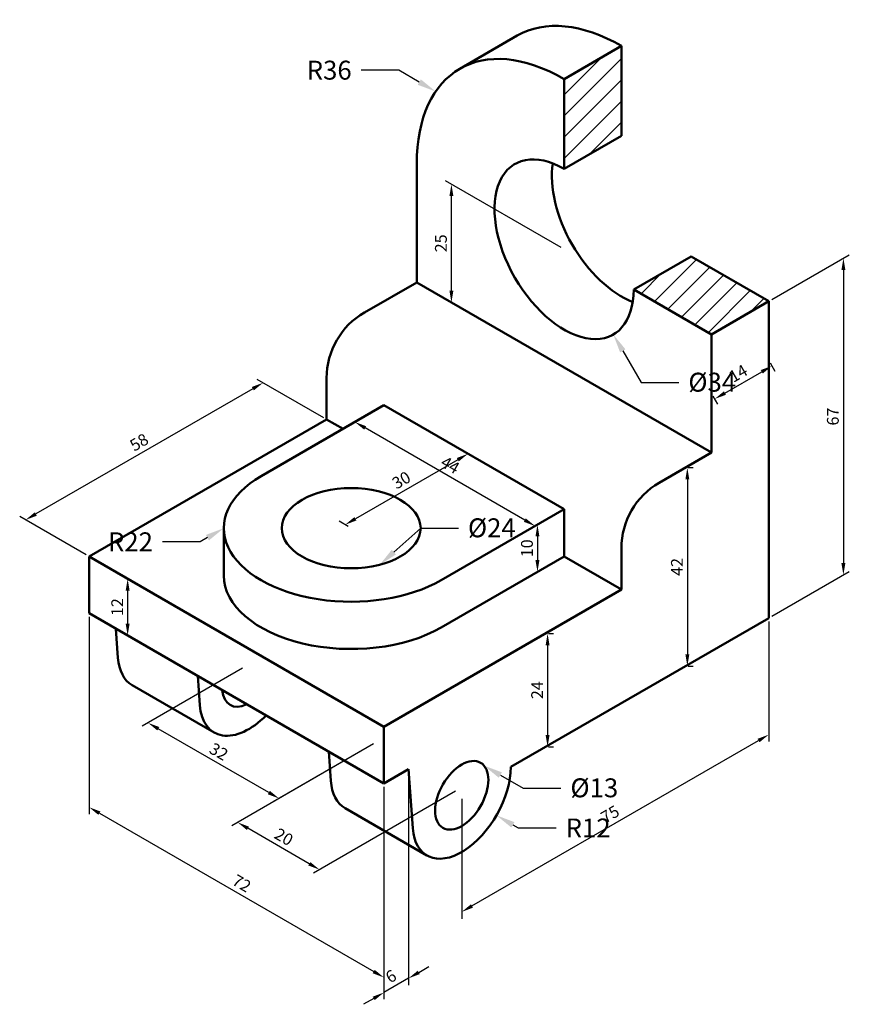
# Model space of a CAD drawing. Units: millimetres. Extents: x 4591 to 4766, y 1465 to 1673.
import ezdxf
from ezdxf import colors
from ezdxf.entities.mleader import LeaderData, LeaderLine
from ezdxf.math import Vec2, Vec3

# ---------------------------------------------------------------- set-up
doc = ezdxf.new("R2010")
doc.units = ezdxf.units.MM
for name, color, linetype, lineweight in [('M-DIMS', 2, 'Continuous', 25), ('M-HATC', 8, 'Continuous', 18), ('M-OUTL', 7, 'Continuous', 50), ('M-TEXT', 3, 'Continuous', 25)]:
    doc.layers.add(name, color=color, linetype=linetype, lineweight=lineweight)
doc.styles.get("Standard").update_dxf_attribs({"font": 'arial.ttf'})
doc.dimstyles.new('ISO-25', dxfattribs={"dimtxt": 2.5, "dimasz": 2.5, "dimexe": 1.25, "dimexo": 0.625, "dimtad": 1, "dimtxsty": 'Standard', "dimcen": 2.5, "dimadec": 0, "dimazin": 0, "dimtfac": 1, "dimtmove": 0, "dimatfit": 3, "dimfxl": 1, "dimarcsym": 0})

# ---------------------------------------------------------------- blocks, each defined once
blk = doc.blocks.new('*D1')
at = {"layer": 'Defpoints', "color": 0, "transparency": 16777216}
for p in [(4749.17, 1546.38), (4749.17, 1521.72), (4684.22, 1508.88)]:
    blk.add_point(p, dxfattribs=at)
at = {"layer": 'M-DIMS', "color": 0, "lineweight": -2, "transparency": 16777216}
for p, q in [((4749.17, 1545.66), (4749.17, 1520.27)), ((4686.39, 1485.47), (4747.01, 1520.47)), ((4684.22, 1508.16), (4684.22, 1482.77))]:
    blk.add_line(p, q, dxfattribs=at)
at = {"layer": 'M-DIMS', "color": 0, "transparency": 16777216}
for points in [[(4746.8, 1520.83), (4747.22, 1520.11), (4749.17, 1521.72)], [(4686.18, 1485.83), (4686.59, 1485.11), (4684.22, 1484.22)]]:
    blk.add_solid(points, dxfattribs=at)
at = {"layer": 'M-DIMS', "color": 0, "transparency": 16777216, "insert": (4715.75, 1504.61), "char_height": 2.5, "attachment_point": 5, "rotation": 30}
blk.add_mtext('75', dxfattribs=at)
blk = doc.blocks.new('*D2')
at = {"layer": 'Defpoints', "color": 0, "transparency": 16777216}
for p in [(4672.96, 1514.38), (4667.77, 1511.38), (4667.77, 1467.17)]:
    blk.add_point(p, dxfattribs=at)
at = {"layer": 'M-DIMS', "color": 0, "lineweight": -2, "transparency": 16777216}
for p, q in [((4672.96, 1513.66), (4672.96, 1468.73)), ((4667.77, 1510.66), (4667.77, 1465.73)), ((4675.13, 1471.42), (4677.29, 1472.67)), ((4672.96, 1470.17), (4667.77, 1467.17)), ((4665.6, 1465.92), (4663.44, 1464.67))]:
    blk.add_line(p, q, dxfattribs=at)
at = {"layer": 'M-DIMS', "color": 0, "transparency": 16777216}
for points in [[(4674.92, 1471.78), (4675.34, 1471.06), (4672.96, 1470.17)], [(4665.39, 1466.28), (4665.81, 1465.56), (4667.77, 1467.17)]]:
    blk.add_solid(points, dxfattribs=at)
at = {"layer": 'M-DIMS', "color": 0, "transparency": 16777216, "insert": (4669.41, 1470.32), "char_height": 2.5, "attachment_point": 5, "rotation": 30}
blk.add_mtext('6', dxfattribs=at)
blk = doc.blocks.new('*D3')
at = {"layer": 'Defpoints', "color": 0, "transparency": 16777216}
for p in [(4655.64, 1588.38), (4591.97, 1567.14), (4605.41, 1559.38)]:
    blk.add_point(p, dxfattribs=at)
at = {"layer": 'M-DIMS', "color": 0, "lineweight": -2, "transparency": 16777216}
for p, q in [((4655.02, 1588.74), (4640.95, 1596.86)), ((4640.04, 1594.89), (4594.14, 1568.39)), ((4604.79, 1559.74), (4590.72, 1567.86))]:
    blk.add_line(p, q, dxfattribs=at)
at = {"layer": 'M-DIMS', "color": 0, "transparency": 16777216}
for points in [[(4639.83, 1595.25), (4640.25, 1594.53), (4642.2, 1596.14)], [(4593.93, 1568.75), (4594.35, 1568.03), (4591.97, 1567.14)]]:
    blk.add_solid(points, dxfattribs=at)
at = {"layer": 'M-DIMS', "color": 0, "transparency": 16777216, "insert": (4616.14, 1583.29), "char_height": 2.5, "attachment_point": 5, "rotation": 30}
blk.add_mtext('58', dxfattribs=at)
blk = doc.blocks.new('*D4')
at = {"layer": 'Defpoints', "color": 0, "transparency": 16777216}
for p in [(4701.94, 1543.12), (4701.94, 1519.12), (4702.38, 1519.12)]:
    blk.add_point(p, dxfattribs=at)
at = {"layer": 'M-DIMS', "color": 0, "lineweight": -2, "transparency": 16777216}
for p, q in [((4702.57, 1543.12), (4703.63, 1543.12)), ((4702.38, 1540.62), (4702.38, 1521.62)), ((4702.57, 1519.12), (4703.63, 1519.12))]:
    blk.add_line(p, q, dxfattribs=at)
at = {"layer": 'M-DIMS', "color": 0, "transparency": 16777216}
for points in [[(4701.96, 1540.62), (4702.79, 1540.62), (4702.38, 1543.12)], [(4701.96, 1521.62), (4702.79, 1521.62), (4702.38, 1519.12)]]:
    blk.add_solid(points, dxfattribs=at)
at = {"layer": 'M-DIMS', "color": 0, "transparency": 16777216, "insert": (4700.5, 1531.12), "char_height": 2.5, "attachment_point": 5, "rotation": 90}
blk.add_mtext('24', dxfattribs=at)
blk = doc.blocks.new('*D5')
at = {"layer": 'Defpoints', "color": 0, "transparency": 16777216}
for p in [(4731.52, 1578.19), (4731.52, 1536.19), (4731.94, 1536.19)]:
    blk.add_point(p, dxfattribs=at)
at = {"layer": 'M-DIMS', "color": 0, "lineweight": -2, "transparency": 16777216}
for p, q in [((4732.15, 1578.19), (4733.19, 1578.19)), ((4731.94, 1575.69), (4731.94, 1538.69)), ((4732.15, 1536.19), (4733.19, 1536.19))]:
    blk.add_line(p, q, dxfattribs=at)
at = {"layer": 'M-DIMS', "color": 0, "transparency": 16777216}
for points in [[(4731.53, 1575.69), (4732.36, 1575.69), (4731.94, 1578.19)], [(4731.53, 1538.69), (4732.36, 1538.69), (4731.94, 1536.19)]]:
    blk.add_solid(points, dxfattribs=at)
at = {"layer": 'M-DIMS', "color": 0, "transparency": 16777216, "insert": (4730.06, 1557.19), "char_height": 2.5, "attachment_point": 5, "rotation": 90}
blk.add_mtext('42', dxfattribs=at)
blk = doc.blocks.new('*D6')
at = {"layer": 'Defpoints', "color": 0, "transparency": 16777216}
for p in [(4749.17, 1613.38), (4764.95, 1555.49), (4749.17, 1546.38)]:
    blk.add_point(p, dxfattribs=at)
at = {"layer": 'M-DIMS', "color": 0, "lineweight": -2, "transparency": 16777216}
for p, q in [((4749.8, 1613.74), (4766.2, 1623.21)), ((4764.95, 1619.99), (4764.95, 1557.99)), ((4749.8, 1546.74), (4766.2, 1556.21))]:
    blk.add_line(p, q, dxfattribs=at)
at = {"layer": 'M-DIMS', "color": 0, "transparency": 16777216}
for points in [[(4764.53, 1619.99), (4765.37, 1619.99), (4764.95, 1622.49)], [(4764.53, 1557.99), (4765.37, 1557.99), (4764.95, 1555.49)]]:
    blk.add_solid(points, dxfattribs=at)
at = {"layer": 'M-DIMS', "color": 0, "transparency": 16777216, "insert": (4763.05, 1588.99), "char_height": 2.5, "attachment_point": 5, "rotation": 90}
blk.add_mtext('67', dxfattribs=at)
blk = doc.blocks.new('*D7')
at = {"layer": 'Defpoints', "color": 0, "transparency": 16777216}
for p in [(4749.17, 1600.88), (4749.85, 1599.72), (4737.05, 1593.88)]:
    blk.add_point(p, dxfattribs=at)
at = {"layer": 'M-DIMS', "color": 0, "lineweight": -2, "transparency": 16777216}
for p, q in [((4749.49, 1600.34), (4750.47, 1598.63)), ((4739.89, 1593.97), (4747.68, 1598.47)), ((4737.36, 1593.34), (4738.35, 1591.63))]:
    blk.add_line(p, q, dxfattribs=at)
at = {"layer": 'M-DIMS', "color": 0, "transparency": 16777216}
for points in [[(4747.47, 1598.83), (4747.89, 1598.1), (4749.85, 1599.72)], [(4739.68, 1594.33), (4740.1, 1593.6), (4737.72, 1592.72)]]:
    blk.add_solid(points, dxfattribs=at)
at = {"layer": 'M-DIMS', "color": 0, "transparency": 16777216, "insert": (4742.85, 1597.84), "char_height": 2.5, "attachment_point": 5, "rotation": 30}
blk.add_mtext('14', dxfattribs=at)
blk = doc.blocks.new('*D8')
at = {"layer": 'Defpoints', "color": 0, "transparency": 16777216}
for p in [(4682.04, 1638.14), (4705.87, 1624.38), (4705.87, 1599.38)]:
    blk.add_point(p, dxfattribs=at)
at = {"layer": 'M-DIMS', "color": 0, "lineweight": -2, "transparency": 16777216}
for p, q in [((4705.25, 1624.74), (4680.79, 1638.86)), ((4682.04, 1615.64), (4682.04, 1635.64)), ((4705.25, 1599.74), (4680.79, 1613.86))]:
    blk.add_line(p, q, dxfattribs=at)
at = {"layer": 'M-DIMS', "color": 0, "transparency": 16777216}
for points in [[(4681.62, 1635.64), (4682.46, 1635.64), (4682.04, 1638.14)], [(4681.62, 1615.64), (4682.46, 1615.64), (4682.04, 1613.14)]]:
    blk.add_solid(points, dxfattribs=at)
at = {"layer": 'M-DIMS', "color": 0, "transparency": 16777216, "insert": (4680.14, 1625.64), "char_height": 2.5, "attachment_point": 5, "rotation": 90}
blk.add_mtext('25', dxfattribs=at)
blk = doc.blocks.new('*D9')
at = {"layer": 'Defpoints', "color": 0, "transparency": 16777216}
for p in [(4667.77, 1591.38), (4661.63, 1587.84), (4705.87, 1569.38)]:
    blk.add_point(p, dxfattribs=at)
at = {"layer": 'M-DIMS', "color": 0, "lineweight": -2, "transparency": 16777216}
for p, q in [((4667.14, 1591.02), (4660.38, 1587.12)), ((4697.57, 1567.09), (4663.8, 1586.59)), ((4705.25, 1569.02), (4698.49, 1565.12))]:
    blk.add_line(p, q, dxfattribs=at)
at = {"layer": 'M-DIMS', "color": 0, "transparency": 16777216}
for points in [[(4664.01, 1586.95), (4663.59, 1586.23), (4661.63, 1587.84)], [(4697.78, 1567.45), (4697.37, 1566.73), (4699.74, 1565.84)]]:
    blk.add_solid(points, dxfattribs=at)
at = {"layer": 'M-DIMS', "color": 0, "transparency": 16777216, "insert": (4681.62, 1578.47), "char_height": 2.5, "attachment_point": 5, "rotation": 330}
blk.add_mtext('44', dxfattribs=at)
blk = doc.blocks.new('*D10')
at = {"layer": 'Defpoints', "color": 0, "transparency": 16777216}
for p in [(4705.87, 1569.38), (4705.87, 1559.38), (4700.24, 1556.13)]:
    blk.add_point(p, dxfattribs=at)
at = {"layer": 'M-DIMS', "color": 0, "lineweight": -2, "transparency": 16777216}
for p, q in [((4705.25, 1569.02), (4698.99, 1565.41)), ((4700.24, 1563.63), (4700.24, 1558.63)), ((4705.25, 1559.02), (4698.99, 1555.41))]:
    blk.add_line(p, q, dxfattribs=at)
at = {"layer": 'M-DIMS', "color": 0, "transparency": 16777216}
for points in [[(4699.82, 1563.63), (4700.65, 1563.63), (4700.24, 1566.13)], [(4699.82, 1558.63), (4700.65, 1558.63), (4700.24, 1556.13)]]:
    blk.add_solid(points, dxfattribs=at)
at = {"layer": 'M-DIMS', "color": 0, "transparency": 16777216, "insert": (4698.34, 1561.13), "char_height": 2.5, "attachment_point": 5, "rotation": 90}
blk.add_mtext('10', dxfattribs=at)
blk = doc.blocks.new('*D11')
at = {"layer": 'Defpoints', "color": 0, "transparency": 16777216}
for p in [(4686.82, 1580.38), (4659.57, 1566.12), (4660.84, 1565.38)]:
    blk.add_point(p, dxfattribs=at)
at = {"layer": 'M-DIMS', "color": 0, "lineweight": -2, "transparency": 16777216}
for p, q in [((4686.19, 1580.74), (4684.3, 1581.84)), ((4683.38, 1579.87), (4661.73, 1567.37)), ((4660.21, 1565.74), (4658.32, 1566.84))]:
    blk.add_line(p, q, dxfattribs=at)
at = {"layer": 'M-DIMS', "color": 0, "transparency": 16777216}
for points in [[(4683.17, 1580.23), (4683.59, 1579.51), (4685.55, 1581.12)], [(4661.52, 1567.73), (4661.94, 1567.01), (4659.57, 1566.12)]]:
    blk.add_solid(points, dxfattribs=at)
at = {"layer": 'M-DIMS', "color": 0, "transparency": 16777216, "insert": (4671.6, 1575.27), "char_height": 2.5, "attachment_point": 5, "rotation": 30}
blk.add_mtext('30', dxfattribs=at)
blk = doc.blocks.new('*D12')
at = {"layer": 'Defpoints', "color": 0, "transparency": 16777216}
for p in [(4605.41, 1547.38), (4667.77, 1511.38), (4667.77, 1470.35)]:
    blk.add_point(p, dxfattribs=at)
at = {"layer": 'M-DIMS', "color": 0, "lineweight": -2, "transparency": 16777216}
for p, q in [((4605.41, 1546.66), (4605.41, 1504.91)), ((4667.77, 1510.66), (4667.77, 1468.91)), ((4607.58, 1505.1), (4665.6, 1471.6))]:
    blk.add_line(p, q, dxfattribs=at)
at = {"layer": 'M-DIMS', "color": 0, "transparency": 16777216}
for points in [[(4607.79, 1505.46), (4607.37, 1504.74), (4605.41, 1506.35)], [(4665.81, 1471.96), (4665.39, 1471.24), (4667.77, 1470.35)]]:
    blk.add_solid(points, dxfattribs=at)
at = {"layer": 'M-DIMS', "color": 0, "transparency": 16777216, "insert": (4637.53, 1489.98), "char_height": 2.5, "attachment_point": 5, "rotation": 330}
blk.add_mtext('72', dxfattribs=at)
blk = doc.blocks.new('*D13')
at = {"layer": 'Defpoints', "color": 0, "transparency": 16777216}
for p in [(4666.19, 1520.11), (4683.52, 1510.11), (4636.83, 1503.15)]:
    blk.add_point(p, dxfattribs=at)
at = {"layer": 'M-DIMS', "color": 0, "lineweight": -2, "transparency": 16777216}
for p, q in [((4665.57, 1519.75), (4635.58, 1502.43)), ((4682.89, 1509.75), (4652.9, 1492.43)), ((4651.98, 1494.4), (4638.99, 1501.9))]:
    blk.add_line(p, q, dxfattribs=at)
at = {"layer": 'M-DIMS', "color": 0, "transparency": 16777216}
for points in [[(4639.2, 1502.26), (4638.78, 1501.54), (4636.83, 1503.15)], [(4652.19, 1494.76), (4651.77, 1494.04), (4654.15, 1493.15)]]:
    blk.add_solid(points, dxfattribs=at)
at = {"layer": 'M-DIMS', "color": 0, "transparency": 16777216, "insert": (4646.44, 1499.8), "char_height": 2.5, "attachment_point": 5, "rotation": 330}
blk.add_mtext('20', dxfattribs=at)
blk = doc.blocks.new('*D14')
at = {"layer": 'Defpoints', "color": 0, "transparency": 16777216}
for p in [(4638.48, 1536.11), (4617.87, 1524.21), (4666.19, 1520.11)]:
    blk.add_point(p, dxfattribs=at)
at = {"layer": 'M-DIMS', "color": 0, "lineweight": -2, "transparency": 16777216}
for p, q in [((4637.86, 1535.75), (4616.62, 1523.49)), ((4643.42, 1509.46), (4620.04, 1522.96)), ((4665.57, 1519.75), (4644.34, 1507.49))]:
    blk.add_line(p, q, dxfattribs=at)
at = {"layer": 'M-DIMS', "color": 0, "transparency": 16777216}
for points in [[(4620.25, 1523.32), (4619.83, 1522.6), (4617.87, 1524.21)], [(4643.63, 1509.82), (4643.21, 1509.1), (4645.59, 1508.21)]]:
    blk.add_solid(points, dxfattribs=at)
at = {"layer": 'M-DIMS', "color": 0, "transparency": 16777216, "insert": (4632.68, 1517.85), "char_height": 2.5, "attachment_point": 5, "rotation": 330}
blk.add_mtext('32', dxfattribs=at)
blk = doc.blocks.new('*D15')
at = {"layer": 'Defpoints', "color": 0, "transparency": 16777216}
for p in [(4621.72, 1549.97), (4613.56, 1542.68), (4621.72, 1537.97)]:
    blk.add_point(p, dxfattribs=at)
at = {"layer": 'M-DIMS', "color": 0, "lineweight": -2, "transparency": 16777216}
for p, q in [((4621.09, 1550.33), (4612.31, 1555.4)), ((4613.56, 1552.18), (4613.56, 1545.18)), ((4621.09, 1538.33), (4612.31, 1543.4))]:
    blk.add_line(p, q, dxfattribs=at)
at = {"layer": 'M-DIMS', "color": 0, "transparency": 16777216}
for points in [[(4613.14, 1552.18), (4613.97, 1552.18), (4613.56, 1554.68)], [(4613.14, 1545.18), (4613.97, 1545.18), (4613.56, 1542.68)]]:
    blk.add_solid(points, dxfattribs=at)
at = {"layer": 'M-DIMS', "color": 0, "transparency": 16777216, "insert": (4611.68, 1548.68), "char_height": 2.5, "attachment_point": 5, "rotation": 90}
blk.add_mtext('12', dxfattribs=at)

msp = doc.modelspace()

# ---------------------------------------------------------------- hatches: boundary and pattern name
at = {"layer": 'M-HATC'}
h = msp.add_hatch(dxfattribs=at)
h.set_pattern_fill('ANSI31', color=256)
h.paths.add_polyline_path([(4717.996, 1667.383), (4705.872, 1660.383), (4705.872, 1641.383), (4717.996, 1648.383)])
h.paths.add_polyline_path([(4749.173, 1613.383), (4732.719, 1622.883), (4720.595, 1615.883), (4737.049, 1606.383)])

# ---------------------------------------------------------------- linework, layer by layer
at = {"layer": 'M-OUTL'}
for p, q in [((4695.951, 1669.567), (4683.827, 1662.567)), ((4705.872, 1660.383), (4717.996, 1667.383)), ((4717.996, 1648.383), (4717.996, 1667.383)), ((4705.872, 1641.383), (4705.872, 1660.383)), ((4705.872, 1641.383), (4717.996, 1648.383)), ((4674.695, 1642.383), (4674.695, 1617.383)), ((4720.595, 1615.883), (4732.719, 1622.883)), ((4732.719, 1622.883), (4749.173, 1613.383)), ((4674.695, 1617.383), (4663.643, 1611.002)), ((4674.695, 1617.383), (4737.049, 1581.383)), ((4720.595, 1615.883), (4737.049, 1606.383)), ((4749.173, 1613.383), (4737.049, 1606.383)), ((4749.173, 1546.383), (4749.173, 1613.383)), ((4737.049, 1606.383), (4737.049, 1581.383)), ((4655.643, 1597.145), (4655.643, 1588.383)), ((4641.786, 1576.383), (4667.767, 1591.383)), ((4705.872, 1569.383), (4667.767, 1591.383)), ((4655.643, 1588.383), (4605.413, 1559.383)), ((4659.107, 1586.383), (4655.643, 1588.383)), ((4737.049, 1581.383), (4725.996, 1575.002)), ((4679.891, 1554.383), (4705.872, 1569.383)), ((4705.872, 1559.383), (4705.872, 1569.383)), ((4633.894, 1565.383), (4633.894, 1555.383)), ((4717.996, 1561.145), (4717.996, 1552.383)), ((4605.413, 1559.383), (4605.413, 1547.383)), ((4605.413, 1559.383), (4667.767, 1523.383)), ((4705.872, 1559.383), (4679.891, 1544.383)), ((4717.996, 1552.383), (4705.872, 1559.383)), ((4717.996, 1552.383), (4667.767, 1523.383)), ((4605.413, 1547.383), (4667.767, 1511.383)), ((4749.173, 1546.383), (4694.614, 1514.883)), ((4611.062, 1544.122), (4611.509, 1537.944)), ((4628.382, 1534.122), (4628.829, 1527.944)), ((4614.519, 1532.155), (4631.84, 1522.155)), ((4667.767, 1523.383), (4667.767, 1511.383)), ((4656.095, 1518.122), (4656.542, 1511.944)), ((4667.767, 1511.383), (4672.963, 1514.383)), ((4672.963, 1514.383), (4673.862, 1501.944)), ((4659.552, 1506.155), (4676.873, 1496.155))]:
    msp.add_line(p, q, dxfattribs=at)
for centre in [(4671.643, 1597.145), (4733.996, 1561.145)]:
    msp.add_arc(centre, 16, 120, 180, dxfattribs=at)
for centre, major_axis, start_param, end_param in [((4717.996, 1631.383), (22.045, -38.184), 8.6393798, 9.424778), ((4705.872, 1624.383), (22.045, -38.184), 8.6393798, 10.2101761), ((4705.872, 1624.383), (10.41, -18.031), 2.3561945, 7.0685835), ((4717.996, 1631.383), (10.41, -18.031), 3.7631762, 5.6616018), ((4660.839, 1565.383), (-26.944, 0), 5.4977871, 8.6393798), ((4660.839, 1555.383), (-26.944, 0), 6.2831853, 8.6393798), ((4621.868, 1544.883), (-7.348, -12.728), 5.5777445, 6.2831853), ((4639.188, 1534.883), (-3.98, -6.894), 5.5780126, 6.988358), ((4639.188, 1534.883), (-7.348, -12.728), 5.5777445, 7.428808), ((4684.221, 1508.883), (-7.348, -12.728), 5.5777445, 8.6393798), ((4666.901, 1518.883), (-7.348, -12.728), 5.5777445, 6.2831853)]:
    msp.add_ellipse(centre, major_axis=major_axis, ratio=0.5773503, start_param=start_param, end_param=end_param, dxfattribs=at)
for centre, major_axis in [((4660.839, 1565.383), (-14.697, 0)), ((4684.221, 1508.883), (-3.98, -6.894))]:
    msp.add_ellipse(centre, major_axis=major_axis, ratio=0.5773503, dxfattribs=at)

# ---------------------------------------------------------------- dimensions: what is measured, and where the dimension line sits
at = {"layer": 'M-DIMS'}
for p1, p2, distance, picture, middle in [((4705.872, 1599.383), (4705.872, 1624.383), 23.832, '*D8', (4680.138, 1625.642)), ((4749.173, 1613.383), (4749.173, 1546.383), 15.775, '*D6', (4763.047, 1588.991)), ((4737.049, 1593.883), (4749.173, 1600.883), -1.348, '*D7', (4742.845, 1597.844)), ((4655.643, 1588.383), (4605.413, 1559.383), -13.441, '*D3', (4616.137, 1583.289)), ((4705.872, 1569.383), (4667.767, 1591.383), 6.133, '*D9', (4681.624, 1578.466)), ((4686.82, 1580.383), (4660.839, 1565.383), -1.273, '*D11', (4671.605, 1575.265)), ((4731.523, 1578.192), (4731.523, 1536.192), 0.421, '*D5', (4730.063, 1557.192)), ((4705.872, 1569.383), (4705.872, 1559.383), -5.635, '*D10', (4698.335, 1561.129)), ((4621.716, 1549.971), (4621.716, 1537.971), -8.16, '*D15', (4611.676, 1548.682)), ((4605.413, 1547.383), (4667.767, 1511.383), -35.536, '*D12', (4637.53, 1489.977)), ((4684.221, 1508.883), (4749.173, 1546.383), -21.361, '*D1', (4715.749, 1504.61)), ((4701.944, 1543.115), (4701.944, 1519.115), 0.434, '*D4', (4700.498, 1531.115)), ((4666.195, 1520.106), (4638.482, 1536.106), 20.609, '*D14', (4632.68, 1517.855)), ((4683.515, 1510.106), (4666.195, 1520.106), 29.368, '*D13', (4646.437, 1499.797)), ((4672.963, 1514.383), (4667.767, 1511.383), 38.288, '*D2', (4669.414, 1470.318))]:
    dim = msp.add_aligned_dim(p1=p1, p2=p2, distance=distance, dimstyle='ISO-25', override={"dimclrd": 0, "dimclre": 0, "dimclrt": 0}, dxfattribs=at)
    dim.commit()
    dim.dimension.update_dxf_attribs({"geometry": picture, "text_midpoint": middle})

# ---------------------------------------------------------------- leaders
at = {"layer": 'M-TEXT'}
ml = msp.add_multileader_mtext('Standard', dxfattribs=at)
ml.set_content('R36', color=256)
ml.set_leader_properties()
ml.build(insert=Vec2(0, 0))
ctx = ml.context
ctx.base_point, ctx.plane_origin = Vec3(4649.389, 1662.232), Vec3(4678.716, 1657.745)
ctx.text_align_type = 2
notes = []
notes.append((ctx, [(0, (1, 1, 0), (4670.944, 1662.232), (-1, 0), 8, [(0, [(4678.716, 1657.745)], 0, [])])]))
ctx.mtext.insert, ctx.mtext.alignment, ctx.mtext.flow_direction = Vec3(4660.944, 1664.267), 3, 5
ml = msp.add_multileader_mtext('Standard', dxfattribs=at)
ml.set_content('%%C34', color=256)
ml.set_leader_properties()
ml.build(insert=Vec2(0, 0))
ctx = ml.context
ctx.base_point, ctx.plane_origin = Vec3(4730.153, 1596.184), Vec3(4716.282, 1606.352)
notes.append((ctx, [(0, (1, 1, 0), (4722.153, 1596.184), (1, 0), 8, [(0, [(4716.282, 1606.352)], 0, [])])]))
ctx.mtext.insert, ctx.mtext.flow_direction = Vec3(4732.153, 1598.265), 5
ml = msp.add_multileader_mtext('Standard', dxfattribs=at)
ml.set_content('%%C24', color=256)
ml.set_leader_properties()
ml.build(insert=Vec2(0, 0))
ctx = ml.context
ctx.base_point, ctx.plane_origin = Vec3(4683.536, 1565.383), Vec3(4666.873, 1557.646)
notes.append((ctx, [(0, (1, 1, 0), (4675.536, 1565.383), (1, 0), 8, [(0, [(4666.873, 1557.646)], 0, [])])]))
ctx.mtext.insert, ctx.mtext.flow_direction = Vec3(4685.536, 1567.463), 5
ml = msp.add_multileader_mtext('Standard', dxfattribs=at)
ml.set_content('R22', color=256)
ml.set_leader_properties()
ml.build(insert=Vec2(0, 0))
ctx = ml.context
ctx.base_point, ctx.plane_origin = Vec3(4607.389, 1562.503), Vec3(4633.894, 1565.383)
ctx.text_align_type = 2
notes.append((ctx, [(0, (1, 1, 0), (4628.906, 1562.503), (-1, 0), 8, [(0, [(4633.894, 1565.383)], 0, [])])]))
ctx.mtext.insert, ctx.mtext.alignment, ctx.mtext.flow_direction = Vec3(4618.906, 1564.503), 3, 5
ml = msp.add_multileader_mtext('Standard', dxfattribs=at)
ml.set_content('%%C13', color=256)
ml.set_leader_properties()
ml.build(insert=Vec2(0, 0))
ctx = ml.context
ctx.base_point, ctx.plane_origin = Vec3(4705.213, 1510.381), Vec3(4688.931, 1515.163)
notes.append((ctx, [(0, (1, 1, 0), (4697.213, 1510.381), (1, 0), 8, [(0, [(4688.931, 1515.163)], 0, [])])]))
ctx.mtext.insert, ctx.mtext.flow_direction = Vec3(4707.213, 1512.462), 5
ml = msp.add_multileader_mtext('Standard', dxfattribs=at)
ml.set_content('R12', color=256)
ml.set_leader_properties()
ml.build(insert=Vec2(0, 0))
ctx = ml.context
ctx.base_point, ctx.plane_origin = Vec3(4704.188, 1501.974), Vec3(4691.57, 1504.64)
notes.append((ctx, [(0, (1, 1, 0), (4696.188, 1501.974), (1, 0), 8, [(0, [(4691.57, 1504.64)], 0, [])])]))
ctx.mtext.insert, ctx.mtext.flow_direction = Vec3(4706.188, 1503.974), 5
for ctx, leaders in notes:
    for number, flags, end, landing, length, lines in leaders:
        leader = LeaderData()
        leader.index, (leader.has_last_leader_line, leader.has_dogleg_vector, leader.attachment_direction) = number, flags
        leader.last_leader_point, leader.dogleg_vector, leader.dogleg_length = Vec3(end), Vec3(landing), length
        for number, points, colour, breaks in lines:
            line = LeaderLine()
            line.index, line.vertices, line.color, line.breaks = number, Vec3.list(points), colors.encode_raw_color(colour), breaks
            leader.lines.append(line)
        ctx.leaders.append(leader)

doc.saveas('drawing.dxf')
